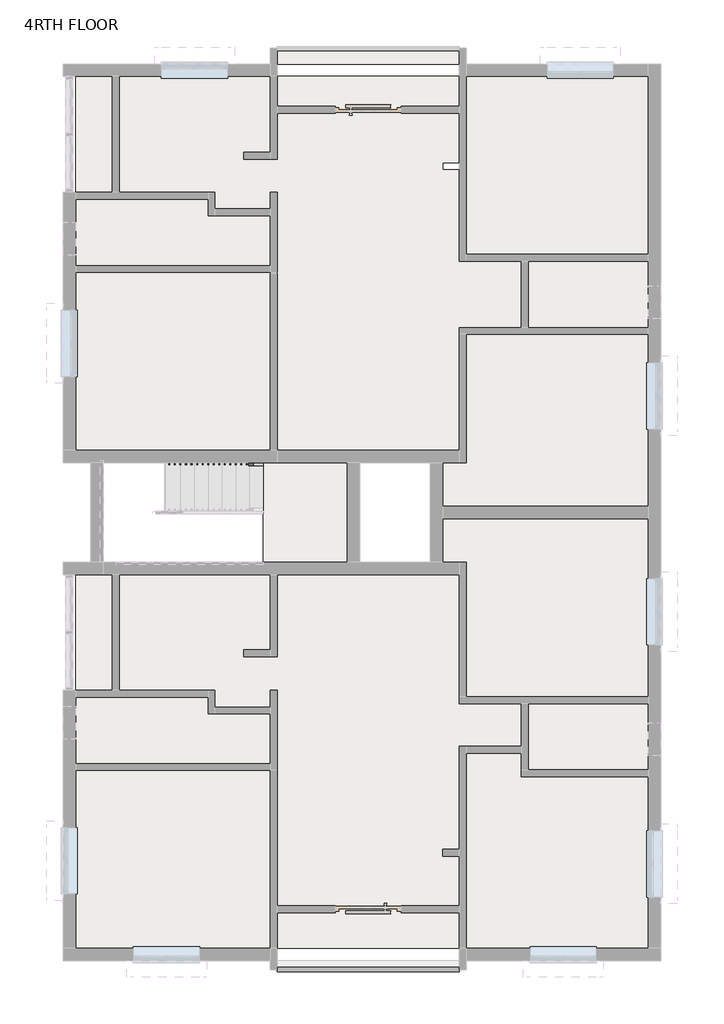
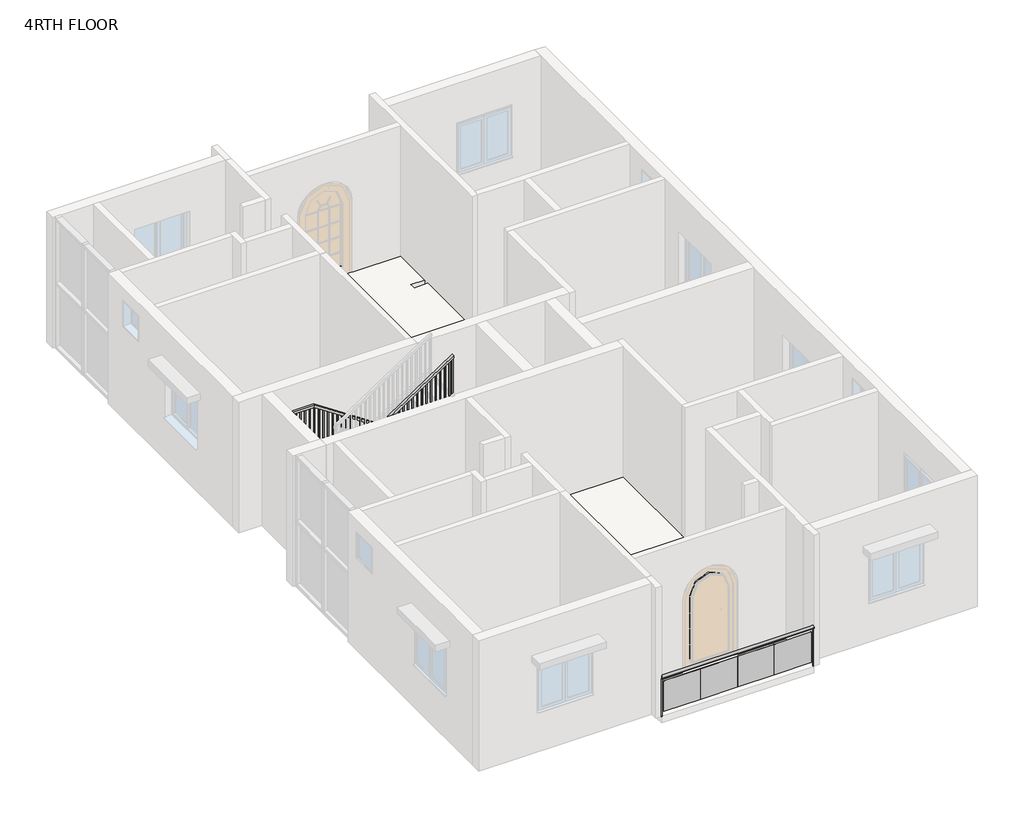
# One storey, part 3 of 4: 5 slabs, 2 railings.
"""IFC4 building model written with IfcOpenShell, lengths in millimetres."""

from ifc_helpers import new_model, si_unit, point, frame, origin, place, context, project, spatial, polyline, ellipse_curve, trimmed, outline, extrude, faceted_brep, element, save
from ifc_brep_helpers import plane_surface, extruded_surface, advanced_brep

model = new_model("IFC4")

# Units and contexts
model_context = context("Model", 3, world=origin())
ifc_project = project(units=[si_unit("LENGTHUNIT", "METRE", prefix="MILLI")], contexts=[model_context])

# Site, building, storey
site = spatial("IfcSite", under=ifc_project)
building = spatial("IfcBuilding", under=site)
storey = spatial("IfcBuildingStorey", under=building, Name="4RTH FLOOR", Elevation=15240.0)

# Railings
placement = place(None, origin())
element("IfcRailing", 1, ObjectType="Glass Panel - Bottom Fill 2", at=placement, inside=storey, context=model_context, shape_type="SolidModel", body=[
    advanced_brep(
    [(-2494.0012202, -3358.1292559, 16154.4), (-2494.0012202, -3434.3292559, 16154.4), (858.7987798, -3358.1292559, 16154.4), (858.7987798, -3434.3292559, 16154.4)],
    [
        (0, 1, ellipse_curve(frame((-2494.0012202, -3396.2292559, 16154.4), z_axis=(-1.0, 0.0, 0.0), x_axis=(0.0, -1.0, 0.0)), 38.1, 28.575)),
        (1, 0, ellipse_curve(frame((-2494.0012202, -3396.2292559, 16154.4), z_axis=(-1.0, 0.0, 0.0), x_axis=(0.0, -1.0, 0.0)), 38.1, 28.575)),
        (2, 3, ellipse_curve(frame((858.7987798, -3396.2292559, 16154.4), z_axis=(1.0, 0.0, 0.0), x_axis=(0.0, -1.0, 0.0)), 38.1, 28.575)),
        (3, 2, ellipse_curve(frame((858.7987798, -3396.2292559, 16154.4), z_axis=(1.0, 0.0, 0.0), x_axis=(0.0, -1.0, 0.0)), 38.1, 28.575)),
        (0, 2),
        (3, 1),
    ],
    [
        plane_surface(frame((-2494.0012202, -3396.2292559, 16154.4), z_axis=(-1.0, 0.0, 0.0), x_axis=(0.0, 1.0, 0.0))),
        plane_surface(frame((858.7987798, -3396.2292559, 16154.4), z_axis=(1.0, 0.0, 0.0), x_axis=(0.0, 1.0, 0.0))),
        extruded_surface(trimmed(ellipse_curve(frame((858.7987798, -3396.2292559, 16154.4), z_axis=(-1.0, 0.0, 0.0), x_axis=(0.0, -1.0, 0.0)), 38.1, 28.575), [point((858.7987798, -3358.1292559, 16154.4))], [point((858.7987798, -3434.3292559, 16154.4))], True, "CARTESIAN"), (-3352.7999999999997, 0.0, 0.0), 3352.7999999999997),
        extruded_surface(trimmed(ellipse_curve(frame((858.7987798, -3396.2292559, 16154.4), z_axis=(-1.0, 0.0, 0.0), x_axis=(0.0, -1.0, 0.0)), 38.1, 28.575), [point((858.7987798, -3434.3292559, 16154.4))], [point((858.7987798, -3358.1292559, 16154.4))], True, "CARTESIAN"), (-3352.7999999999997, 0.0, 0.0), 3352.7999999999997),
    ],
    [
        (0, [[1, 2]]),
        (1, [[3, 4]]),
        (2, [[-1, 5, -4, 6]]),
        (3, [[-2, -6, -3, -5]]),
    ],
),
    extrude(outline(polyline([(-4.8012202, -3402.7644129), (-4.8012202, -3396.4144129), (807.9987798, -3396.4144129), (807.9987798, -3402.7644129), (-4.8012202, -3402.7644129)])), frame((0.0, 0.0, 15341.6), z_axis=(0.0, 0.0, 1.0), x_axis=(1.0, 0.0, 0.0)), (0.0, 0.0, 1.0), 711.2),
    extrude(outline(polyline([(-817.6012202, -3402.7644129), (-817.6012202, -3396.4144129), (-4.8012202, -3396.4144129), (-4.8012202, -3402.7644129), (-817.6012202, -3402.7644129)])), frame((0.0, 0.0, 15341.6), z_axis=(0.0, 0.0, 1.0), x_axis=(1.0, 0.0, 0.0)), (0.0, 0.0, 1.0), 711.2),
    extrude(outline(polyline([(-1630.4012202, -3402.7644129), (-1630.4012202, -3396.4144129), (-817.6012202, -3396.4144129), (-817.6012202, -3402.7644129), (-1630.4012202, -3402.7644129)])), frame((0.0, 0.0, 15341.6), z_axis=(0.0, 0.0, 1.0), x_axis=(1.0, 0.0, 0.0)), (0.0, 0.0, 1.0), 711.2),
    extrude(outline(polyline([(-2443.2012202, -3402.7644129), (-2443.2012202, -3396.4144129), (-1630.4012202, -3396.4144129), (-1630.4012202, -3402.7644129), (-2443.2012202, -3402.7644129)])), frame((0.0, 0.0, 15341.6), z_axis=(0.0, 0.0, 1.0), x_axis=(1.0, 0.0, 0.0)), (0.0, 0.0, 1.0), 711.2),
    extrude(outline(polyline([(846.0987798, -3386.7042559), (865.1487798, -3386.7042559), (865.1487798, -3405.7542559), (846.0987798, -3405.7542559), (846.0987798, -3386.7042559)])), frame((0.0, 0.0, 15240.0), z_axis=(0.0, 0.0, 1.0), x_axis=(1.0, 0.0, 0.0)), (0.0, 0.0, 1.0), 885.825),
    extrude(outline(polyline([(-2500.3512202, -3386.7042559), (-2481.3012202, -3386.7042559), (-2481.3012202, -3405.7542559), (-2500.3512202, -3405.7542559), (-2500.3512202, -3386.7042559)])), frame((0.0, 0.0, 15240.0), z_axis=(0.0, 0.0, 1.0), x_axis=(1.0, 0.0, 0.0)), (0.0, 0.0, 1.0), 885.825),
])
element("IfcRailing", 2, ObjectType="Handrail - Rectangular", at=placement, inside=storey, context=model_context, shape_type="SolidModel", body=[
    faceted_brep([(-2748.0012202, 5879.8309003, 16323.7333333), (-2748.0012202, 5879.8309003, 16262.6793317), (-2748.0012202, 5930.6309003, 16262.6793317), (-2748.0012202, 5930.6309003, 16323.7333333), (-4780.0012202, 5879.8309003, 17678.4), (-4795.3822226, 5879.8309003, 17627.6), (-4795.3822226, 5930.6309003, 17627.6), (-4780.0012202, 5930.6309003, 17678.4), (-5643.6012202, 5879.8309003, 17678.4), (-5643.6012202, 5879.8309003, 17627.6), (-5694.4012202, 5930.6309003, 17627.6), (-5694.4012202, 5930.6309003, 17678.4), (-5643.6012202, 4152.6309003, 17678.4), (-5643.6012202, 4152.6309003, 17627.6), (-5694.4012202, 4101.8309003, 17627.6), (-5694.4012202, 4101.8309003, 17678.4), (-5034.0012202, 4152.6309003, 17678.4), (-5018.6202178, 4152.6309003, 17627.6), (-5018.6202178, 4101.8309003, 17627.6), (-5034.0012202, 4101.8309003, 17678.4), (-2748.0012202, 4152.6309003, 19202.4), (-2748.0012202, 4101.8309003, 19202.4), (-2748.0012202, 4101.8309003, 19141.3459984), (-2748.0012202, 4152.6309003, 19141.3459984)], [[[0, 1, 2, 3]], [[1, 0, 4, 5]], [[2, 1, 5, 6]], [[3, 2, 6, 7]], [[0, 3, 7, 4]], [[5, 4, 8, 9]], [[6, 5, 9, 10]], [[7, 6, 10, 11]], [[4, 7, 11, 8]], [[9, 8, 12, 13]], [[10, 9, 13, 14]], [[11, 10, 14, 15]], [[8, 11, 15, 12]], [[13, 12, 16, 17]], [[14, 13, 17, 18]], [[15, 14, 18, 19]], [[12, 15, 19, 16]], [[20, 21, 22, 23]], [[17, 16, 20, 23]], [[18, 17, 23, 22]], [[19, 18, 22, 21]], [[16, 19, 21, 20]]]),
    extrude(outline(polyline([(19096.8959984, -2814.6762202), (19084.1959984, -2833.7262202), (18118.6666667, -2833.7262202), (18118.6666667, -2814.6762202), (19096.8959984, -2814.6762202)])), frame((0.0, 4117.7059003, 0.0), z_axis=(0.0, 1.0, 0.0), x_axis=(0.0, 0.0, 1.0)), (0.0, 0.0, 1.0), 19.05),
    extrude(outline(polyline([(19029.1626651, -2916.2762202), (19016.4626651, -2935.3262202), (18118.6666667, -2935.3262202), (18118.6666667, -2916.2762202), (19029.1626651, -2916.2762202)])), frame((0.0, 4117.7059003, 0.0), z_axis=(0.0, 1.0, 0.0), x_axis=(0.0, 0.0, 1.0)), (0.0, 0.0, 1.0), 19.05),
    extrude(outline(polyline([(18961.4293317, -3017.8762202), (18948.7293317, -3036.9262202), (17949.3333333, -3036.9262202), (17949.3333333, -3017.8762202), (18961.4293317, -3017.8762202)])), frame((0.0, 4117.7059003, 0.0), z_axis=(0.0, 1.0, 0.0), x_axis=(0.0, 0.0, 1.0)), (0.0, 0.0, 1.0), 19.05),
    extrude(outline(polyline([(18893.6959984, -3119.4762202), (18880.9959984, -3138.5262202), (17949.3333333, -3138.5262202), (17949.3333333, -3119.4762202), (18893.6959984, -3119.4762202)])), frame((0.0, 4117.7059003, 0.0), z_axis=(0.0, 1.0, 0.0), x_axis=(0.0, 0.0, 1.0)), (0.0, 0.0, 1.0), 19.05),
    extrude(outline(polyline([(18825.9626651, -3221.0762202), (18813.2626651, -3240.1262202), (17949.3333333, -3240.1262202), (17949.3333333, -3221.0762202), (18825.9626651, -3221.0762202)])), frame((0.0, 4117.7059003, 0.0), z_axis=(0.0, 1.0, 0.0), x_axis=(0.0, 0.0, 1.0)), (0.0, 0.0, 1.0), 19.05),
    extrude(outline(polyline([(18758.2293317, -3322.6762202), (18745.5293317, -3341.7262202), (17780.0, -3341.7262202), (17780.0, -3322.6762202), (18758.2293317, -3322.6762202)])), frame((0.0, 4117.7059003, 0.0), z_axis=(0.0, 1.0, 0.0), x_axis=(0.0, 0.0, 1.0)), (0.0, 0.0, 1.0), 19.05),
    extrude(outline(polyline([(18690.4959984, -3424.2762202), (18677.7959984, -3443.3262202), (17780.0, -3443.3262202), (17780.0, -3424.2762202), (18690.4959984, -3424.2762202)])), frame((0.0, 4117.7059003, 0.0), z_axis=(0.0, 1.0, 0.0), x_axis=(0.0, 0.0, 1.0)), (0.0, 0.0, 1.0), 19.05),
    extrude(outline(polyline([(18622.7626651, -3525.8762202), (18610.0626651, -3544.9262202), (17610.6666667, -3544.9262202), (17610.6666667, -3525.8762202), (18622.7626651, -3525.8762202)])), frame((0.0, 4117.7059003, 0.0), z_axis=(0.0, 1.0, 0.0), x_axis=(0.0, 0.0, 1.0)), (0.0, 0.0, 1.0), 19.05),
    extrude(outline(polyline([(18555.0293317, -3627.4762202), (18542.3293317, -3646.5262202), (17610.6666667, -3646.5262202), (17610.6666667, -3627.4762202), (18555.0293317, -3627.4762202)])), frame((0.0, 4117.7059003, 0.0), z_axis=(0.0, 1.0, 0.0), x_axis=(0.0, 0.0, 1.0)), (0.0, 0.0, 1.0), 19.05),
    extrude(outline(polyline([(18487.2959984, -3729.0762202), (18474.5959984, -3748.1262202), (17610.6666667, -3748.1262202), (17610.6666667, -3729.0762202), (18487.2959984, -3729.0762202)])), frame((0.0, 4117.7059003, 0.0), z_axis=(0.0, 1.0, 0.0), x_axis=(0.0, 0.0, 1.0)), (0.0, 0.0, 1.0), 19.05),
    extrude(outline(polyline([(18419.5626651, -3830.6762202), (18406.8626651, -3849.7262202), (17441.3333333, -3849.7262202), (17441.3333333, -3830.6762202), (18419.5626651, -3830.6762202)])), frame((0.0, 4117.7059003, 0.0), z_axis=(0.0, 1.0, 0.0), x_axis=(0.0, 0.0, 1.0)), (0.0, 0.0, 1.0), 19.05),
    extrude(outline(polyline([(18351.8293317, -3932.2762202), (18339.1293317, -3951.3262202), (17441.3333333, -3951.3262202), (17441.3333333, -3932.2762202), (18351.8293317, -3932.2762202)])), frame((0.0, 4117.7059003, 0.0), z_axis=(0.0, 1.0, 0.0), x_axis=(0.0, 0.0, 1.0)), (0.0, 0.0, 1.0), 19.05),
    extrude(outline(polyline([(18284.0959984, -4033.8762202), (18271.3959984, -4052.9262202), (17272.0, -4052.9262202), (17272.0, -4033.8762202), (18284.0959984, -4033.8762202)])), frame((0.0, 4117.7059003, 0.0), z_axis=(0.0, 1.0, 0.0), x_axis=(0.0, 0.0, 1.0)), (0.0, 0.0, 1.0), 19.05),
    extrude(outline(polyline([(18216.3626651, -4135.4762202), (18203.6626651, -4154.5262202), (17272.0, -4154.5262202), (17272.0, -4135.4762202), (18216.3626651, -4135.4762202)])), frame((0.0, 4117.7059003, 0.0), z_axis=(0.0, 1.0, 0.0), x_axis=(0.0, 0.0, 1.0)), (0.0, 0.0, 1.0), 19.05),
    extrude(outline(polyline([(18148.6293317, -4237.0762202), (18135.9293317, -4256.1262202), (17272.0, -4256.1262202), (17272.0, -4237.0762202), (18148.6293317, -4237.0762202)])), frame((0.0, 4117.7059003, 0.0), z_axis=(0.0, 1.0, 0.0), x_axis=(0.0, 0.0, 1.0)), (0.0, 0.0, 1.0), 19.05),
    extrude(outline(polyline([(18080.8959984, -4338.6762202), (18068.1959984, -4357.7262202), (17102.6666667, -4357.7262202), (17102.6666667, -4338.6762202), (18080.8959984, -4338.6762202)])), frame((0.0, 4117.7059003, 0.0), z_axis=(0.0, 1.0, 0.0), x_axis=(0.0, 0.0, 1.0)), (0.0, 0.0, 1.0), 19.05),
    extrude(outline(polyline([(18013.1626651, -4440.2762202), (18000.4626651, -4459.3262202), (17102.6666667, -4459.3262202), (17102.6666667, -4440.2762202), (18013.1626651, -4440.2762202)])), frame((0.0, 4117.7059003, 0.0), z_axis=(0.0, 1.0, 0.0), x_axis=(0.0, 0.0, 1.0)), (0.0, 0.0, 1.0), 19.05),
    extrude(outline(polyline([(17945.4293317, -4541.8762202), (17932.7293317, -4560.9262202), (16933.3333333, -4560.9262202), (16933.3333333, -4541.8762202), (17945.4293317, -4541.8762202)])), frame((0.0, 4117.7059003, 0.0), z_axis=(0.0, 1.0, 0.0), x_axis=(0.0, 0.0, 1.0)), (0.0, 0.0, 1.0), 19.05),
    extrude(outline(polyline([(17877.6959984, -4643.4762202), (17864.9959984, -4662.5262202), (16933.3333333, -4662.5262202), (16933.3333333, -4643.4762202), (17877.6959984, -4643.4762202)])), frame((0.0, 4117.7059003, 0.0), z_axis=(0.0, 1.0, 0.0), x_axis=(0.0, 0.0, 1.0)), (0.0, 0.0, 1.0), 19.05),
    extrude(outline(polyline([(17809.9626651, -4745.0762202), (17797.2626651, -4764.1262202), (16933.3333333, -4764.1262202), (16933.3333333, -4745.0762202), (17809.9626651, -4745.0762202)])), frame((0.0, 4117.7059003, 0.0), z_axis=(0.0, 1.0, 0.0), x_axis=(0.0, 0.0, 1.0)), (0.0, 0.0, 1.0), 19.05),
    extrude(outline(polyline([(17742.2293317, -4846.6762202), (17729.5293317, -4865.7262202), (16764.0, -4865.7262202), (16764.0, -4846.6762202), (17742.2293317, -4846.6762202)])), frame((0.0, 4117.7059003, 0.0), z_axis=(0.0, 1.0, 0.0), x_axis=(0.0, 0.0, 1.0)), (0.0, 0.0, 1.0), 19.05),
    extrude(outline(polyline([(17674.4959984, -4948.2762202), (17661.7959984, -4967.3262202), (16764.0, -4967.3262202), (16764.0, -4948.2762202), (17674.4959984, -4948.2762202)])), frame((0.0, 4117.7059003, 0.0), z_axis=(0.0, 1.0, 0.0), x_axis=(0.0, 0.0, 1.0)), (0.0, 0.0, 1.0), 19.05),
    extrude(outline(polyline([(-5068.9262202, 4117.7059003), (-5068.9262202, 4136.7559003), (-5049.8762202, 4136.7559003), (-5049.8762202, 4117.7059003), (-5068.9262202, 4117.7059003)])), frame((0.0, 0.0, 16764.0), z_axis=(0.0, 0.0, 1.0), x_axis=(1.0, 0.0, 0.0)), (0.0, 0.0, 1.0), 863.6),
    extrude(outline(polyline([(-5170.5262202, 4117.7059003), (-5170.5262202, 4136.7559003), (-5151.4762202, 4136.7559003), (-5151.4762202, 4117.7059003), (-5170.5262202, 4117.7059003)])), frame((0.0, 0.0, 16764.0), z_axis=(0.0, 0.0, 1.0), x_axis=(1.0, 0.0, 0.0)), (0.0, 0.0, 1.0), 863.6),
    extrude(outline(polyline([(-5272.1262202, 4117.7059003), (-5272.1262202, 4136.7559003), (-5253.0762202, 4136.7559003), (-5253.0762202, 4117.7059003), (-5272.1262202, 4117.7059003)])), frame((0.0, 0.0, 16764.0), z_axis=(0.0, 0.0, 1.0), x_axis=(1.0, 0.0, 0.0)), (0.0, 0.0, 1.0), 863.6),
    extrude(outline(polyline([(-5373.7262202, 4117.7059003), (-5373.7262202, 4136.7559003), (-5354.6762202, 4136.7559003), (-5354.6762202, 4117.7059003), (-5373.7262202, 4117.7059003)])), frame((0.0, 0.0, 16764.0), z_axis=(0.0, 0.0, 1.0), x_axis=(1.0, 0.0, 0.0)), (0.0, 0.0, 1.0), 863.6),
    extrude(outline(polyline([(-5475.3262202, 4117.7059003), (-5475.3262202, 4136.7559003), (-5456.2762202, 4136.7559003), (-5456.2762202, 4117.7059003), (-5475.3262202, 4117.7059003)])), frame((0.0, 0.0, 16764.0), z_axis=(0.0, 0.0, 1.0), x_axis=(1.0, 0.0, 0.0)), (0.0, 0.0, 1.0), 863.6),
    extrude(outline(polyline([(-5576.9262202, 4117.7059003), (-5576.9262202, 4136.7559003), (-5557.8762202, 4136.7559003), (-5557.8762202, 4117.7059003), (-5576.9262202, 4117.7059003)])), frame((0.0, 0.0, 16764.0), z_axis=(0.0, 0.0, 1.0), x_axis=(1.0, 0.0, 0.0)), (0.0, 0.0, 1.0), 863.6),
    extrude(outline(polyline([(-5678.5262202, 4187.5559003), (-5659.4762202, 4187.5559003), (-5659.4762202, 4168.5059003), (-5678.5262202, 4168.5059003), (-5678.5262202, 4187.5559003)])), frame((0.0, 0.0, 16764.0), z_axis=(0.0, 0.0, 1.0), x_axis=(1.0, 0.0, 0.0)), (0.0, 0.0, 1.0), 863.6),
    extrude(outline(polyline([(-5678.5262202, 4289.1559003), (-5659.4762202, 4289.1559003), (-5659.4762202, 4270.1059003), (-5678.5262202, 4270.1059003), (-5678.5262202, 4289.1559003)])), frame((0.0, 0.0, 16764.0), z_axis=(0.0, 0.0, 1.0), x_axis=(1.0, 0.0, 0.0)), (0.0, 0.0, 1.0), 863.6),
    extrude(outline(polyline([(-5678.5262202, 4390.7559003), (-5659.4762202, 4390.7559003), (-5659.4762202, 4371.7059003), (-5678.5262202, 4371.7059003), (-5678.5262202, 4390.7559003)])), frame((0.0, 0.0, 16764.0), z_axis=(0.0, 0.0, 1.0), x_axis=(1.0, 0.0, 0.0)), (0.0, 0.0, 1.0), 863.6),
    extrude(outline(polyline([(-5678.5262202, 4492.3559003), (-5659.4762202, 4492.3559003), (-5659.4762202, 4473.3059003), (-5678.5262202, 4473.3059003), (-5678.5262202, 4492.3559003)])), frame((0.0, 0.0, 16764.0), z_axis=(0.0, 0.0, 1.0), x_axis=(1.0, 0.0, 0.0)), (0.0, 0.0, 1.0), 863.6),
    extrude(outline(polyline([(-5678.5262202, 4593.9559003), (-5659.4762202, 4593.9559003), (-5659.4762202, 4574.9059003), (-5678.5262202, 4574.9059003), (-5678.5262202, 4593.9559003)])), frame((0.0, 0.0, 16764.0), z_axis=(0.0, 0.0, 1.0), x_axis=(1.0, 0.0, 0.0)), (0.0, 0.0, 1.0), 863.6),
    extrude(outline(polyline([(-5678.5262202, 4695.5559003), (-5659.4762202, 4695.5559003), (-5659.4762202, 4676.5059003), (-5678.5262202, 4676.5059003), (-5678.5262202, 4695.5559003)])), frame((0.0, 0.0, 16764.0), z_axis=(0.0, 0.0, 1.0), x_axis=(1.0, 0.0, 0.0)), (0.0, 0.0, 1.0), 863.6),
    extrude(outline(polyline([(-5678.5262202, 4797.1559003), (-5659.4762202, 4797.1559003), (-5659.4762202, 4778.1059003), (-5678.5262202, 4778.1059003), (-5678.5262202, 4797.1559003)])), frame((0.0, 0.0, 16764.0), z_axis=(0.0, 0.0, 1.0), x_axis=(1.0, 0.0, 0.0)), (0.0, 0.0, 1.0), 863.6),
    extrude(outline(polyline([(-5678.5262202, 4898.7559003), (-5659.4762202, 4898.7559003), (-5659.4762202, 4879.7059003), (-5678.5262202, 4879.7059003), (-5678.5262202, 4898.7559003)])), frame((0.0, 0.0, 16764.0), z_axis=(0.0, 0.0, 1.0), x_axis=(1.0, 0.0, 0.0)), (0.0, 0.0, 1.0), 863.6),
    extrude(outline(polyline([(-5678.5262202, 5000.3559003), (-5659.4762202, 5000.3559003), (-5659.4762202, 4981.3059003), (-5678.5262202, 4981.3059003), (-5678.5262202, 5000.3559003)])), frame((0.0, 0.0, 16764.0), z_axis=(0.0, 0.0, 1.0), x_axis=(1.0, 0.0, 0.0)), (0.0, 0.0, 1.0), 863.6),
    extrude(outline(polyline([(-5678.5262202, 5101.9559003), (-5659.4762202, 5101.9559003), (-5659.4762202, 5082.9059003), (-5678.5262202, 5082.9059003), (-5678.5262202, 5101.9559003)])), frame((0.0, 0.0, 16764.0), z_axis=(0.0, 0.0, 1.0), x_axis=(1.0, 0.0, 0.0)), (0.0, 0.0, 1.0), 863.6),
    extrude(outline(polyline([(-5678.5262202, 5203.5559003), (-5659.4762202, 5203.5559003), (-5659.4762202, 5184.5059003), (-5678.5262202, 5184.5059003), (-5678.5262202, 5203.5559003)])), frame((0.0, 0.0, 16764.0), z_axis=(0.0, 0.0, 1.0), x_axis=(1.0, 0.0, 0.0)), (0.0, 0.0, 1.0), 863.6),
    extrude(outline(polyline([(-5678.5262202, 5305.1559003), (-5659.4762202, 5305.1559003), (-5659.4762202, 5286.1059003), (-5678.5262202, 5286.1059003), (-5678.5262202, 5305.1559003)])), frame((0.0, 0.0, 16764.0), z_axis=(0.0, 0.0, 1.0), x_axis=(1.0, 0.0, 0.0)), (0.0, 0.0, 1.0), 863.6),
    extrude(outline(polyline([(-5678.5262202, 5406.7559003), (-5659.4762202, 5406.7559003), (-5659.4762202, 5387.7059003), (-5678.5262202, 5387.7059003), (-5678.5262202, 5406.7559003)])), frame((0.0, 0.0, 16764.0), z_axis=(0.0, 0.0, 1.0), x_axis=(1.0, 0.0, 0.0)), (0.0, 0.0, 1.0), 863.6),
    extrude(outline(polyline([(-5678.5262202, 5508.3559003), (-5659.4762202, 5508.3559003), (-5659.4762202, 5489.3059003), (-5678.5262202, 5489.3059003), (-5678.5262202, 5508.3559003)])), frame((0.0, 0.0, 16764.0), z_axis=(0.0, 0.0, 1.0), x_axis=(1.0, 0.0, 0.0)), (0.0, 0.0, 1.0), 863.6),
    extrude(outline(polyline([(-5678.5262202, 5609.9559003), (-5659.4762202, 5609.9559003), (-5659.4762202, 5590.9059003), (-5678.5262202, 5590.9059003), (-5678.5262202, 5609.9559003)])), frame((0.0, 0.0, 16764.0), z_axis=(0.0, 0.0, 1.0), x_axis=(1.0, 0.0, 0.0)), (0.0, 0.0, 1.0), 863.6),
    extrude(outline(polyline([(-5678.5262202, 5711.5559003), (-5659.4762202, 5711.5559003), (-5659.4762202, 5692.5059003), (-5678.5262202, 5692.5059003), (-5678.5262202, 5711.5559003)])), frame((0.0, 0.0, 16764.0), z_axis=(0.0, 0.0, 1.0), x_axis=(1.0, 0.0, 0.0)), (0.0, 0.0, 1.0), 863.6),
    extrude(outline(polyline([(-5678.5262202, 5813.1559003), (-5659.4762202, 5813.1559003), (-5659.4762202, 5794.1059003), (-5678.5262202, 5794.1059003), (-5678.5262202, 5813.1559003)])), frame((0.0, 0.0, 16764.0), z_axis=(0.0, 0.0, 1.0), x_axis=(1.0, 0.0, 0.0)), (0.0, 0.0, 1.0), 863.6),
    extrude(outline(polyline([(-5583.2762202, 5914.7559003), (-5583.2762202, 5895.7059003), (-5602.3262202, 5895.7059003), (-5602.3262202, 5914.7559003), (-5583.2762202, 5914.7559003)])), frame((0.0, 0.0, 16764.0), z_axis=(0.0, 0.0, 1.0), x_axis=(1.0, 0.0, 0.0)), (0.0, 0.0, 1.0), 863.6),
    extrude(outline(polyline([(-5481.6762202, 5914.7559003), (-5481.6762202, 5895.7059003), (-5500.7262202, 5895.7059003), (-5500.7262202, 5914.7559003), (-5481.6762202, 5914.7559003)])), frame((0.0, 0.0, 16764.0), z_axis=(0.0, 0.0, 1.0), x_axis=(1.0, 0.0, 0.0)), (0.0, 0.0, 1.0), 863.6),
    extrude(outline(polyline([(-5380.0762202, 5914.7559003), (-5380.0762202, 5895.7059003), (-5399.1262202, 5895.7059003), (-5399.1262202, 5914.7559003), (-5380.0762202, 5914.7559003)])), frame((0.0, 0.0, 16764.0), z_axis=(0.0, 0.0, 1.0), x_axis=(1.0, 0.0, 0.0)), (0.0, 0.0, 1.0), 863.6),
    extrude(outline(polyline([(-5278.4762202, 5914.7559003), (-5278.4762202, 5895.7059003), (-5297.5262202, 5895.7059003), (-5297.5262202, 5914.7559003), (-5278.4762202, 5914.7559003)])), frame((0.0, 0.0, 16764.0), z_axis=(0.0, 0.0, 1.0), x_axis=(1.0, 0.0, 0.0)), (0.0, 0.0, 1.0), 863.6),
    extrude(outline(polyline([(-5176.8762202, 5914.7559003), (-5176.8762202, 5895.7059003), (-5195.9262202, 5895.7059003), (-5195.9262202, 5914.7559003), (-5176.8762202, 5914.7559003)])), frame((0.0, 0.0, 16764.0), z_axis=(0.0, 0.0, 1.0), x_axis=(1.0, 0.0, 0.0)), (0.0, 0.0, 1.0), 863.6),
    extrude(outline(polyline([(-5075.2762202, 5914.7559003), (-5075.2762202, 5895.7059003), (-5094.3262202, 5895.7059003), (-5094.3262202, 5914.7559003), (-5075.2762202, 5914.7559003)])), frame((0.0, 0.0, 16764.0), z_axis=(0.0, 0.0, 1.0), x_axis=(1.0, 0.0, 0.0)), (0.0, 0.0, 1.0), 863.6),
    extrude(outline(polyline([(-4973.6762202, 5914.7559003), (-4973.6762202, 5895.7059003), (-4992.7262202, 5895.7059003), (-4992.7262202, 5914.7559003), (-4973.6762202, 5914.7559003)])), frame((0.0, 0.0, 16764.0), z_axis=(0.0, 0.0, 1.0), x_axis=(1.0, 0.0, 0.0)), (0.0, 0.0, 1.0), 863.6),
    extrude(outline(polyline([(-4872.0762202, 5914.7559003), (-4872.0762202, 5895.7059003), (-4891.1262202, 5895.7059003), (-4891.1262202, 5914.7559003), (-4872.0762202, 5914.7559003)])), frame((0.0, 0.0, 16764.0), z_axis=(0.0, 0.0, 1.0), x_axis=(1.0, 0.0, 0.0)), (0.0, 0.0, 1.0), 863.6),
    extrude(outline(polyline([(17610.9959984, -4770.4762202), (17623.6959984, -4789.5262202), (16764.0, -4789.5262202), (16764.0, -4770.4762202), (17610.9959984, -4770.4762202)])), frame((0.0, 5895.7059003, 0.0), z_axis=(0.0, 1.0, 0.0), x_axis=(0.0, 0.0, 1.0)), (0.0, 0.0, 1.0), 19.05),
    extrude(outline(polyline([(17543.2626651, -4668.8762202), (17555.9626651, -4687.9262202), (16594.6666667, -4687.9262202), (16594.6666667, -4668.8762202), (17543.2626651, -4668.8762202)])), frame((0.0, 5895.7059003, 0.0), z_axis=(0.0, 1.0, 0.0), x_axis=(0.0, 0.0, 1.0)), (0.0, 0.0, 1.0), 19.05),
    extrude(outline(polyline([(17475.5293317, -4567.2762202), (17488.2293317, -4586.3262202), (16594.6666667, -4586.3262202), (16594.6666667, -4567.2762202), (17475.5293317, -4567.2762202)])), frame((0.0, 5895.7059003, 0.0), z_axis=(0.0, 1.0, 0.0), x_axis=(0.0, 0.0, 1.0)), (0.0, 0.0, 1.0), 19.05),
    extrude(outline(polyline([(17407.7959984, -4465.6762202), (17420.4959984, -4484.7262202), (16425.3333333, -4484.7262202), (16425.3333333, -4465.6762202), (17407.7959984, -4465.6762202)])), frame((0.0, 5895.7059003, 0.0), z_axis=(0.0, 1.0, 0.0), x_axis=(0.0, 0.0, 1.0)), (0.0, 0.0, 1.0), 19.05),
    extrude(outline(polyline([(17340.0626651, -4364.0762202), (17352.7626651, -4383.1262202), (16425.3333333, -4383.1262202), (16425.3333333, -4364.0762202), (17340.0626651, -4364.0762202)])), frame((0.0, 5895.7059003, 0.0), z_axis=(0.0, 1.0, 0.0), x_axis=(0.0, 0.0, 1.0)), (0.0, 0.0, 1.0), 19.05),
    extrude(outline(polyline([(17272.3293317, -4262.4762202), (17285.0293317, -4281.5262202), (16425.3333333, -4281.5262202), (16425.3333333, -4262.4762202), (17272.3293317, -4262.4762202)])), frame((0.0, 5895.7059003, 0.0), z_axis=(0.0, 1.0, 0.0), x_axis=(0.0, 0.0, 1.0)), (0.0, 0.0, 1.0), 19.05),
    extrude(outline(polyline([(17204.5959984, -4160.8762202), (17217.2959984, -4179.9262202), (16256.0, -4179.9262202), (16256.0, -4160.8762202), (17204.5959984, -4160.8762202)])), frame((0.0, 5895.7059003, 0.0), z_axis=(0.0, 1.0, 0.0), x_axis=(0.0, 0.0, 1.0)), (0.0, 0.0, 1.0), 19.05),
    extrude(outline(polyline([(17136.8626651, -4059.2762202), (17149.5626651, -4078.3262202), (16256.0, -4078.3262202), (16256.0, -4059.2762202), (17136.8626651, -4059.2762202)])), frame((0.0, 5895.7059003, 0.0), z_axis=(0.0, 1.0, 0.0), x_axis=(0.0, 0.0, 1.0)), (0.0, 0.0, 1.0), 19.05),
    extrude(outline(polyline([(17069.1293317, -3957.6762202), (17081.8293317, -3976.7262202), (16086.6666667, -3976.7262202), (16086.6666667, -3957.6762202), (17069.1293317, -3957.6762202)])), frame((0.0, 5895.7059003, 0.0), z_axis=(0.0, 1.0, 0.0), x_axis=(0.0, 0.0, 1.0)), (0.0, 0.0, 1.0), 19.05),
    extrude(outline(polyline([(17001.3959984, -3856.0762202), (17014.0959984, -3875.1262202), (16086.6666667, -3875.1262202), (16086.6666667, -3856.0762202), (17001.3959984, -3856.0762202)])), frame((0.0, 5895.7059003, 0.0), z_axis=(0.0, 1.0, 0.0), x_axis=(0.0, 0.0, 1.0)), (0.0, 0.0, 1.0), 19.05),
    extrude(outline(polyline([(16933.6626651, -3754.4762202), (16946.3626651, -3773.5262202), (16086.6666667, -3773.5262202), (16086.6666667, -3754.4762202), (16933.6626651, -3754.4762202)])), frame((0.0, 5895.7059003, 0.0), z_axis=(0.0, 1.0, 0.0), x_axis=(0.0, 0.0, 1.0)), (0.0, 0.0, 1.0), 19.05),
    extrude(outline(polyline([(16865.9293317, -3652.8762202), (16878.6293317, -3671.9262202), (15917.3333333, -3671.9262202), (15917.3333333, -3652.8762202), (16865.9293317, -3652.8762202)])), frame((0.0, 5895.7059003, 0.0), z_axis=(0.0, 1.0, 0.0), x_axis=(0.0, 0.0, 1.0)), (0.0, 0.0, 1.0), 19.05),
    extrude(outline(polyline([(16798.1959984, -3551.2762202), (16810.8959984, -3570.3262202), (15917.3333333, -3570.3262202), (15917.3333333, -3551.2762202), (16798.1959984, -3551.2762202)])), frame((0.0, 5895.7059003, 0.0), z_axis=(0.0, 1.0, 0.0), x_axis=(0.0, 0.0, 1.0)), (0.0, 0.0, 1.0), 19.05),
    extrude(outline(polyline([(16730.4626651, -3449.6762202), (16743.1626651, -3468.7262202), (15748.0, -3468.7262202), (15748.0, -3449.6762202), (16730.4626651, -3449.6762202)])), frame((0.0, 5895.7059003, 0.0), z_axis=(0.0, 1.0, 0.0), x_axis=(0.0, 0.0, 1.0)), (0.0, 0.0, 1.0), 19.05),
    extrude(outline(polyline([(16662.7293317, -3348.0762202), (16675.4293317, -3367.1262202), (15748.0, -3367.1262202), (15748.0, -3348.0762202), (16662.7293317, -3348.0762202)])), frame((0.0, 5895.7059003, 0.0), z_axis=(0.0, 1.0, 0.0), x_axis=(0.0, 0.0, 1.0)), (0.0, 0.0, 1.0), 19.05),
    extrude(outline(polyline([(16594.9959984, -3246.4762202), (16607.6959984, -3265.5262202), (15748.0, -3265.5262202), (15748.0, -3246.4762202), (16594.9959984, -3246.4762202)])), frame((0.0, 5895.7059003, 0.0), z_axis=(0.0, 1.0, 0.0), x_axis=(0.0, 0.0, 1.0)), (0.0, 0.0, 1.0), 19.05),
    extrude(outline(polyline([(16527.2626651, -3144.8762202), (16539.9626651, -3163.9262202), (15578.6666667, -3163.9262202), (15578.6666667, -3144.8762202), (16527.2626651, -3144.8762202)])), frame((0.0, 5895.7059003, 0.0), z_axis=(0.0, 1.0, 0.0), x_axis=(0.0, 0.0, 1.0)), (0.0, 0.0, 1.0), 19.05),
    extrude(outline(polyline([(16459.5293317, -3043.2762202), (16472.2293317, -3062.3262202), (15578.6666667, -3062.3262202), (15578.6666667, -3043.2762202), (16459.5293317, -3043.2762202)])), frame((0.0, 5895.7059003, 0.0), z_axis=(0.0, 1.0, 0.0), x_axis=(0.0, 0.0, 1.0)), (0.0, 0.0, 1.0), 19.05),
    extrude(outline(polyline([(16391.7959984, -2941.6762202), (16404.4959984, -2960.7262202), (15409.3333333, -2960.7262202), (15409.3333333, -2941.6762202), (16391.7959984, -2941.6762202)])), frame((0.0, 5895.7059003, 0.0), z_axis=(0.0, 1.0, 0.0), x_axis=(0.0, 0.0, 1.0)), (0.0, 0.0, 1.0), 19.05),
    extrude(outline(polyline([(16324.0626651, -2840.0762202), (16336.7626651, -2859.1262202), (15409.3333333, -2859.1262202), (15409.3333333, -2840.0762202), (16324.0626651, -2840.0762202)])), frame((0.0, 5895.7059003, 0.0), z_axis=(0.0, 1.0, 0.0), x_axis=(0.0, 0.0, 1.0)), (0.0, 0.0, 1.0), 19.05),
    extrude(outline(polyline([(-5678.5262202, 4136.7559003), (-5659.4762202, 4136.7559003), (-5659.4762202, 4117.7059003), (-5678.5262202, 4117.7059003), (-5678.5262202, 4136.7559003)])), frame((0.0, 0.0, 16764.0), z_axis=(0.0, 0.0, 1.0), x_axis=(1.0, 0.0, 0.0)), (0.0, 0.0, 1.0), 863.6),
    extrude(outline(polyline([(-5659.4762202, 5914.7559003), (-5659.4762202, 5895.7059003), (-5678.5262202, 5895.7059003), (-5678.5262202, 5914.7559003), (-5659.4762202, 5914.7559003)])), frame((0.0, 0.0, 16764.0), z_axis=(0.0, 0.0, 1.0), x_axis=(1.0, 0.0, 0.0)), (0.0, 0.0, 1.0), 863.6),
    extrude(outline(polyline([(19141.3459984, -2748.0012202), (19128.6459984, -2767.0512202), (18118.6666667, -2767.0512202), (18118.6666667, -2748.0012202), (19141.3459984, -2748.0012202)])), frame((0.0, 4117.7059003, 0.0), z_axis=(0.0, 1.0, 0.0), x_axis=(0.0, 0.0, 1.0)), (0.0, 0.0, 1.0), 19.05),
    extrude(outline(polyline([(16262.6793317, -2748.0012202), (16275.3793317, -2767.0512202), (15409.3333333, -2767.0512202), (15409.3333333, -2748.0012202), (16262.6793317, -2748.0012202)])), frame((0.0, 5895.7059003, 0.0), z_axis=(0.0, 1.0, 0.0), x_axis=(0.0, 0.0, 1.0)), (0.0, 0.0, 1.0), 19.05),
])

# Slabs
element("IfcSlab", 3, ObjectType="FLOORING 6\"", at=placement, inside=storey, context=model_context, shape_type="SweptSolid", body=[
    extrude(outline(polyline([(-2621.0012202, 11645.6309003), (-3103.6012202, 11645.6309003), (-3103.6012202, 11518.6309003), (-2557.5012202, 11518.6309003), (-2494.0012202, 11518.6309003), (-2494.0012202, 13042.6309003), (858.7987798, 13042.6309003), (858.7987798, 11455.1309003), (553.9987798, 11455.1309003), (553.9987798, 11328.1309003), (858.7987798, 11328.1309003), (858.7987798, 9639.0309003), (2001.7987798, 9639.0309003), (2001.7987798, 8419.8309003), (858.7987798, 8419.8309003), (858.7987798, 6159.2309003), (-2494.0012202, 6159.2309003), (-2494.0012202, 9435.8309003), (-2494.0012202, 10909.0309003), (-2621.0012202, 10909.0309003), (-2621.0012202, 10604.2309003), (-3637.0012202, 10604.2309003), (-3637.0012202, 10909.0309003), (-6202.4012202, 10909.0309003), (-6202.4012202, 13042.6309003), (-2621.0012202, 13042.6309003), (-2621.0012202, 11645.6309003)])), frame((0.0, 0.0, 15087.6), z_axis=(0.0, 0.0, 1.0), x_axis=(1.0, 0.0, 0.0)), (0.0, 0.0, 1.0), 152.4),
])
element("IfcSlab", 4, ObjectType="FLOORING 6\"", at=placement, inside=storey, context=model_context, shape_type="SweptSolid", body=[
    extrude(outline(polyline([(4338.5987798, 13042.6309003), (4338.5987798, 9766.0309003), (985.7987798, 9766.0309003), (985.7987798, 13042.6309003), (4338.5987798, 13042.6309003)])), frame((0.0, 0.0, 15087.6), z_axis=(0.0, 0.0, 1.0), x_axis=(1.0, 0.0, 0.0)), (0.0, 0.0, 1.0), 152.4),
    extrude(outline(polyline([(4338.5987798, 9639.0309003), (4338.5987798, 8419.8309003), (2128.7987798, 8419.8309003), (2128.7987798, 9639.0309003), (4338.5987798, 9639.0309003)])), frame((0.0, 0.0, 15087.6), z_axis=(0.0, 0.0, 1.0), x_axis=(1.0, 0.0, 0.0)), (0.0, 0.0, 1.0), 152.4),
    extrude(outline(polyline([(-2621.0012202, 9435.8309003), (-2621.0012202, 6159.2309003), (-6202.4012202, 6159.2309003), (-6202.4012202, 9435.8309003), (-2621.0012202, 9435.8309003)])), frame((0.0, 0.0, 15087.6), z_axis=(0.0, 0.0, 1.0), x_axis=(1.0, 0.0, 0.0)), (0.0, 0.0, 1.0), 152.4),
    extrude(outline(polyline([(-2621.0012202, 9562.8309003), (-6202.4012202, 9562.8309003), (-6202.4012202, 10782.0309003), (-3764.0012202, 10782.0309003), (-3764.0012202, 10477.2309003), (-2621.0012202, 10477.2309003), (-2621.0012202, 9562.8309003)])), frame((0.0, 0.0, 15087.6), z_axis=(0.0, 0.0, 1.0), x_axis=(1.0, 0.0, 0.0)), (0.0, 0.0, 1.0), 152.4),
    extrude(outline(polyline([(553.9987798, 5930.6309003), (985.7987798, 5930.6309003), (985.7987798, 8292.8309003), (4338.5987798, 8292.8309003), (4338.5987798, 5130.5309003), (553.9987798, 5130.5309003), (553.9987798, 5930.6309003)])), frame((0.0, 0.0, 15087.6), z_axis=(0.0, 0.0, 1.0), x_axis=(1.0, 0.0, 0.0)), (0.0, 0.0, 1.0), 152.4),
])
element("IfcSlab", 5, ObjectType="FLOORING 6\"", at=placement, inside=storey, context=model_context, shape_type="SweptSolid", body=[
    extrude(outline(polyline([(985.7987798, 583.9309003), (2001.7987798, 583.9309003), (2001.7987798, 152.1309003), (4338.5987798, 152.1309003), (4338.5987798, -3010.1690997), (985.7987798, -3010.1690997), (985.7987798, 583.9309003)])), frame((0.0, 0.0, 15087.6), z_axis=(0.0, 0.0, 1.0), x_axis=(1.0, 0.0, 0.0)), (0.0, 0.0, 1.0), 152.4),
    extrude(outline(polyline([(-6203.9887202, -3010.1690997), (-6203.9887202, 266.4309003), (-2621.0012202, 266.4309003), (-2621.0012202, -3010.1690997), (-6203.9887202, -3010.1690997)])), frame((0.0, 0.0, 15087.6), z_axis=(0.0, 0.0, 1.0), x_axis=(1.0, 0.0, 0.0)), (0.0, 0.0, 1.0), 152.4),
    extrude(outline(polyline([(-2621.0012202, 393.4309003), (-6203.9887202, 393.4309003), (-6203.9887202, 1612.6309003), (-3764.0012202, 1612.6309003), (-3764.0012202, 1307.8309003), (-2621.0012202, 1307.8309003), (-2621.0012202, 393.4309003)])), frame((0.0, 0.0, 15087.6), z_axis=(0.0, 0.0, 1.0), x_axis=(1.0, 0.0, 0.0)), (0.0, 0.0, 1.0), 152.4),
    extrude(outline(polyline([(858.7987798, -3010.1690997), (-2494.0012202, -3010.1690997), (-2494.0012202, 1739.6309003), (-2621.0012202, 1739.6309003), (-2621.0012202, 1434.8309003), (-3637.0012202, 1434.8309003), (-3637.0012202, 1739.6309003), (-6203.9887202, 1739.6309003), (-6203.9887202, 3873.2309003), (-2621.0012202, 3873.2309003), (-2621.0012202, 2488.9309003), (-3103.6012202, 2488.9309003), (-3103.6012202, 2361.9309003), (-2494.0012202, 2361.9309003), (-2494.0012202, 3873.2309003), (858.7987798, 3873.2309003), (858.7987798, 1498.3309003), (2001.7987798, 1498.3309003), (2001.7987798, 710.9309003), (858.7987798, 710.9309003), (858.7987798, -3010.1690997)])), frame((0.0, 0.0, 15087.6), z_axis=(0.0, 0.0, 1.0), x_axis=(1.0, 0.0, 0.0)), (0.0, 0.0, 1.0), 152.4),
    extrude(outline(polyline([(985.7987798, 1625.3309003), (985.7987798, 4101.8309003), (553.9987798, 4101.8309003), (553.9987798, 4901.9309003), (4338.5987798, 4901.9309003), (4338.5987798, 1625.3309003), (985.7987798, 1625.3309003)])), frame((0.0, 0.0, 15087.6), z_axis=(0.0, 0.0, 1.0), x_axis=(1.0, 0.0, 0.0)), (0.0, 0.0, 1.0), 152.4),
    extrude(outline(polyline([(-2748.0012202, 4000.2309003), (-2748.0012202, 5981.4309003), (-2748.0012202, 6032.2309003), (-2494.0012202, 6032.2309003), (-2494.0012202, 5930.6309003), (-1198.6012202, 5930.6309003), (-1198.6012202, 4101.8309003), (-2494.0012202, 4101.8309003), (-2494.0012202, 4000.2309003), (-2748.0012202, 4000.2309003)])), frame((0.0, 0.0, 15087.6), z_axis=(0.0, 0.0, 1.0), x_axis=(1.0, 0.0, 0.0)), (0.0, 0.0, 1.0), 152.4),
])
element("IfcSlab", 6, ObjectType="bathroom tiles", at=placement, inside=storey, context=model_context, shape_type="SweptSolid", body=[
    extrude(outline(polyline([(858.7987798, 13563.3309003), (858.7987798, 13271.2309003), (-2494.0012202, 13271.2309003), (-2494.0012202, 13563.3309003), (858.7987798, 13563.3309003)])), frame((0.0, 0.0, 15087.6), z_axis=(0.0, 0.0, 1.0), x_axis=(1.0, 0.0, 0.0)), (0.0, 0.0, 1.0), 152.4),
])
element("IfcSlab", 7, ObjectType="bathroom tiles", at=placement, inside=storey, context=model_context, shape_type="SweptSolid", body=[
    extrude(outline(polyline([(4338.5987798, 1498.3309003), (4338.5987798, 279.1309003), (2128.7987798, 279.1309003), (2128.7987798, 1498.3309003), (4338.5987798, 1498.3309003)])), frame((0.0, 0.0, 15087.6), z_axis=(0.0, 0.0, 1.0), x_axis=(1.0, 0.0, 0.0)), (0.0, 0.0, 1.0), 152.4),
])

save(model, "model.ifc")

# Revit data of these elements
# Type "Glass Panel - Bottom Fill 2"
#   Assembly Code = "C2010400"
#   built-in parameter 1008612 = 0.0416667 (stored number, unit not read)
#   built-in parameter 1008611 = 0.0416667 (stored number, unit not read)
#   built-in parameter 1008609 = 0.333333 (stored number, unit not read)
#   built-in parameter 1008604 = 0.166667 (stored number, unit not read)
#   built-in parameter 1008603 = 0.166667 (stored number, unit not read)
#   Railing Height = 3' - 0"
#   built-in parameter 1008630 = 2
#   built-in parameter 1008610 = 2
#   built-in parameter 1008618 = Baluster - Square : 3/4"
# Type "Handrail - Rectangular"
#   Assembly Code = "C2010400"
#   built-in parameter 1008612 = 0.0416667 (stored number, unit not read)
#   built-in parameter 1008611 = 0.0416667 (stored number, unit not read)
#   built-in parameter 1008609 = 0.333333 (stored number, unit not read)
#   built-in parameter 1008604 = 0.166667 (stored number, unit not read)
#   built-in parameter 1008603 = 0.166667 (stored number, unit not read)
#   Railing Height = 3' - 0"
#   built-in parameter 1008630 = 2
#   built-in parameter 1008610 = 2
#   built-in parameter 1008618 = Baluster - Square : 3/4"
# Type "FLOORING 6\""
#   Assembly Code = "B1010"
#   Function = 0
#   Layers, outside or top first: 0' - 6" "MARBLE FLOORING" (function 1)
# Type "bathroom tiles"
#   Assembly Code = "B1010"
#   Function = 0
#   Layers, outside or top first: 0' - 6" "tile flooring" (function 1)
# Element 1 (IfcRailing, "Glass Panel - Bottom Fill 2")
#   Phase Created = New Construction
#   Materials on its faces: "Glass"
# Element 2 (IfcRailing, "Handrail - Rectangular")
#   Phase Created = New Construction
# Element 3 (IfcSlab, "FLOORING 6\"")
#   built-in parameter 1001955 = -1.5708 (stored number, unit not read)
#   Height Offset From Level = 0' - 0"
#   Phase Created = New Construction
#   Materials on its faces: "MARBLE FLOORING"
# Element 4 (IfcSlab, "FLOORING 6\"")
#   Height Offset From Level = 0' - 0"
#   Phase Created = New Construction
#   Materials on its faces: "MARBLE FLOORING"
# Element 5 (IfcSlab, "FLOORING 6\"")
#   built-in parameter 1001955 = 1.5708 (stored number, unit not read)
#   Height Offset From Level = 0' - 0"
#   Phase Created = New Construction
#   Materials on its faces: "MARBLE FLOORING"
# Elements 6, 7 (IfcSlab, "bathroom tiles")
#   Height Offset From Level = 0' - 0"
#   Phase Created = New Construction
#   Materials on its faces: "tile flooring"
# Materials
#   "MARBLE FLOORING": class "Generic", colour RGB 120 120 120, transparency 0, Cost = 0
#   "tile flooring": class "Generic", colour RGB 120 120 120, transparency 0, Cost = 0
#   "Glass": class "Glass", colour RGB 0 128 192, transparency 0.75, Description = "Soda Lime Glass", Cost = 0
